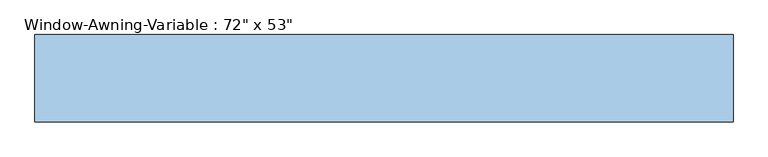
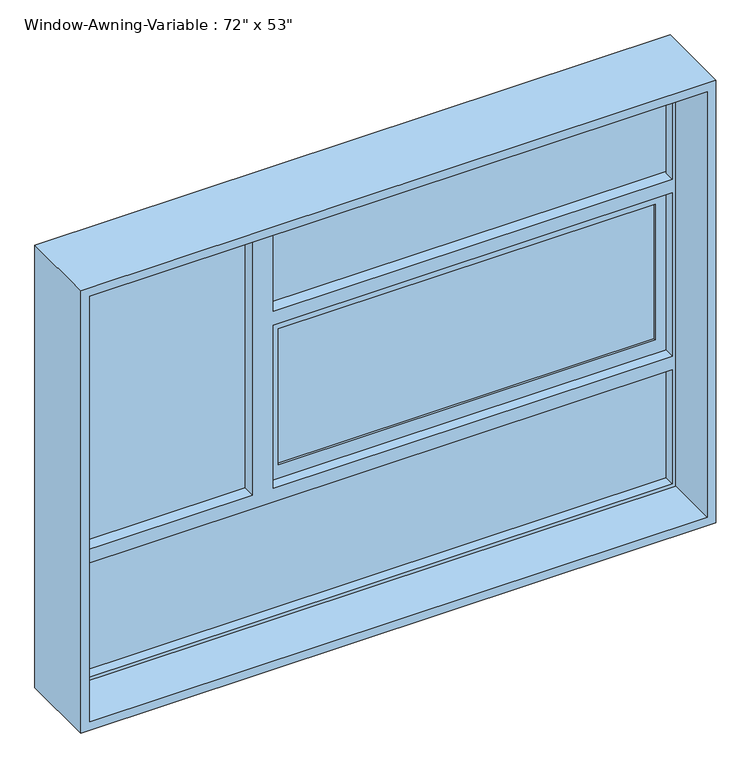
"""IFC4 building model written with IfcOpenShell, lengths in millimetres: window geometry."""

from ifc_helpers import new_model, si_unit, frame, origin, place, context, project, spatial, polyline, outline, extrude, faceted_brep, source, transform, mapped, element, save


def window_dd9b4f56(model_context):
    return source(origin(), model_context, "Body", "SolidModel", [
        extrude(outline(polyline([(847.1296875, 98.425), (847.1296875, 92.075), (-237.5296875, 92.075), (-237.5296875, 98.425), (847.1296875, 98.425)])), frame((0.0, 0.0, 1381.0654688), z_axis=(0.0, 0.0, 1.0), x_axis=(1.0, 0.0, 0.0)), (0.0, 0.0, 1.0), 412.8690625),
        extrude(outline(polyline([(847.1296875, 85.725), (847.1296875, 79.375), (-237.5296875, 79.375), (-237.5296875, 85.725), (847.1296875, 85.725)])), frame((0.0, 0.0, 1381.0654688), z_axis=(0.0, 0.0, 1.0), x_axis=(1.0, 0.0, 0.0)), (0.0, 0.0, 1.0), 412.8690625),
        extrude(outline(polyline([(-330.2, 98.425), (-330.2, 92.075), (-889.0, 92.075), (-889.0, 98.425), (-330.2, 98.425)])), frame((0.0, 0.0, 1339.1951563), z_axis=(0.0, 0.0, 1.0), x_axis=(1.0, 0.0, 0.0)), (0.0, 0.0, 1.0), 896.0048438),
        extrude(outline(polyline([(-330.2, 85.725), (-330.2, 79.375), (-889.0, 79.375), (-889.0, 85.725), (-330.2, 85.725)])), frame((0.0, 0.0, 1339.1951563), z_axis=(0.0, 0.0, 1.0), x_axis=(1.0, 0.0, 0.0)), (0.0, 0.0, 1.0), 896.0048438),
        extrude(outline(polyline([(889.0, 85.725), (889.0, 79.375), (-279.4, 79.375), (-279.4, 85.725), (889.0, 85.725)])), frame((0.0, 0.0, 1877.6751563), z_axis=(0.0, 0.0, 1.0), x_axis=(1.0, 0.0, 0.0)), (0.0, 0.0, 1.0), 357.5248438),
        extrude(outline(polyline([(889.0, 98.425), (889.0, 92.075), (-279.4, 92.075), (-279.4, 98.425), (889.0, 98.425)])), frame((0.0, 0.0, 1877.6751563), z_axis=(0.0, 0.0, 1.0), x_axis=(1.0, 0.0, 0.0)), (0.0, 0.0, 1.0), 357.5248438),
        extrude(outline(polyline([(889.0, 98.425), (889.0, 92.075), (-889.0, 92.075), (-889.0, 98.425), (889.0, 98.425)])), frame((0.0, 0.0, 939.8), z_axis=(0.0, 0.0, 1.0), x_axis=(1.0, 0.0, 0.0)), (0.0, 0.0, 1.0), 357.5248438),
        extrude(outline(polyline([(889.0, 85.725), (889.0, 79.375), (-889.0, 79.375), (-889.0, 85.725), (889.0, 85.725)])), frame((0.0, 0.0, 939.8), z_axis=(0.0, 0.0, 1.0), x_axis=(1.0, 0.0, 0.0)), (0.0, 0.0, 1.0), 357.5248438),
        faceted_brep([(-889.0, 73.025, 2235.2), (-889.0, 114.3, 2235.2), (889.0, 114.3, 2235.2), (889.0, 73.025, 2235.2), (-279.4, 73.025, 2235.2), (-279.4, 111.125, 2235.2), (-330.2, 111.125, 2235.2), (-330.2, 73.025, 2235.2), (-878.8796875, 42.06875, 2225.0796875), (-878.8796875, 73.025, 2225.0796875), (-330.2, 73.025, 2225.0796875), (-330.2, 42.06875, 2225.0796875), (878.8796875, 73.025, 2225.0796875), (878.8796875, 42.06875, 2225.0796875), (-269.2796875, 42.06875, 2225.0796875), (-269.2796875, 73.025, 2225.0796875), (-889.0, -114.3, 2235.2), (-889.0, 42.06875, 2235.2), (889.0, 42.06875, 2235.2), (889.0, -114.3, 2235.2), (-914.4, 114.3, 2260.6), (-914.4, -114.3, 2260.6), (914.4, -114.3, 2260.6), (914.4, 114.3, 2260.6), (889.0, 114.3, 939.8), (889.0, 73.025, 939.8), (889.0, 73.025, 1297.3248438), (889.0, 111.125, 1297.3248438), (889.0, 111.125, 1339.1951563), (889.0, 73.025, 1339.1951563), (889.0, 73.025, 1835.8048438), (889.0, 111.125, 1835.8048438), (889.0, 111.125, 1877.6751563), (889.0, 73.025, 1877.6751563), (878.8796875, 73.025, 1877.6751563), (878.8796875, 42.06875, 1877.6751563), (878.8796875, 73.025, 949.9203125), (878.8796875, 42.06875, 949.9203125), (878.8796875, 42.06875, 1297.3248438), (878.8796875, 73.025, 1297.3248438), (878.8796875, 73.025, 1339.1951563), (878.8796875, 42.06875, 1339.1951563), (878.8796875, 42.06875, 1835.8048438), (878.8796875, 73.025, 1835.8048438), (889.0, 42.06875, 939.8), (889.0, -114.3, 939.8), (914.4, -114.3, 914.4), (914.4, 114.3, 914.4), (-889.0, 114.3, 939.8), (-889.0, 73.025, 939.8), (-878.8796875, 73.025, 949.9203125), (-878.8796875, 42.06875, 949.9203125), (-889.0, 42.06875, 939.8), (-889.0, -114.3, 939.8), (-914.4, -114.3, 914.4), (-914.4, 114.3, 914.4), (-889.0, 73.025, 1339.1951563), (-889.0, 111.125, 1339.1951563), (-889.0, 111.125, 1297.3248438), (-889.0, 73.025, 1297.3248438), (-269.2796875, 73.025, 1877.6751563), (-279.4, 73.025, 1877.6751563), (-878.8796875, 73.025, 1297.3248438), (-878.8796875, 73.025, 1339.1951563), (-269.2796875, 73.025, 1339.1951563), (-279.4, 73.025, 1339.1951563), (-279.4, 73.025, 1835.8048438), (-269.2796875, 73.025, 1835.8048438), (-878.8796875, 42.06875, 1339.1951563), (-878.8796875, 42.06875, 1297.3248438), (-269.2796875, 42.06875, 1877.6751563), (-330.2, 42.06875, 1339.1951563), (-269.2796875, 42.06875, 1339.1951563), (-269.2796875, 42.06875, 1835.8048438), (-330.2, 111.125, 1339.1951563), (-279.4, 111.125, 1877.6751563), (-279.4, 111.125, 1835.8048438), (-279.4, 111.125, 1339.1951563)], [[[0, 1, 2, 3, 4, 5, 6, 7]], [[8, 9, 10, 11]], [[12, 13, 14, 15]], [[16, 17, 18, 19]], [[20, 21, 22, 23]], [[3, 2, 24, 25, 26, 27, 28, 29, 30, 31, 32, 33]], [[13, 12, 34, 35]], [[36, 37, 38, 39]], [[40, 41, 42, 43]], [[19, 18, 44, 45]], [[23, 22, 46, 47]], [[25, 24, 48, 49]], [[37, 36, 50, 51]], [[45, 44, 52, 53]], [[47, 46, 54, 55]], [[1, 0, 56, 57, 58, 59, 49, 48]], [[12, 15, 60, 61, 4, 3, 33, 34]], [[25, 49, 59, 62, 50, 36, 39, 26]], [[56, 0, 7, 10, 9, 63]], [[29, 40, 43, 30]], [[64, 65, 66, 67]], [[9, 8, 68, 63]], [[51, 50, 62, 69]], [[52, 44, 18, 17], [14, 13, 35, 70], [37, 51, 69, 38], [68, 8, 11, 71], [72, 73, 42, 41]], [[17, 16, 53, 52]], [[22, 21, 54, 46], [16, 19, 45, 53]], [[21, 20, 55, 54]], [[20, 23, 47, 55], [2, 1, 48, 24]], [[58, 27, 26, 39, 38, 69, 62, 59]], [[27, 58, 57, 74, 6, 5, 75, 32, 31, 76, 77, 28]], [[29, 28, 77, 65, 64, 72, 41, 40]], [[57, 56, 63, 68, 71, 74]], [[6, 74, 71, 11, 10, 7]], [[15, 14, 70, 60]], [[72, 64, 67, 73]], [[5, 4, 61, 75]], [[65, 77, 76, 66]], [[76, 31, 30, 43, 42, 73, 67, 66]], [[32, 75, 61, 60, 70, 35, 34, 33]]]),
        extrude(outline(polyline([(1339.1951563, -279.4), (1339.1951563, 889.0), (1835.8048438, 889.0), (1835.8048438, -279.4), (1339.1951563, -279.4)]), holes=[polyline([(1381.0654688, -237.5296875), (1793.9345313, -237.5296875), (1793.9345313, 847.1296875), (1381.0654688, 847.1296875), (1381.0654688, -237.5296875)])]), frame((0.0, 73.025, 0.0), z_axis=(0.0, 1.0, 0.0), x_axis=(0.0, 0.0, 1.0)), (0.0, 0.0, 1.0), 31.75),
    ])


if __name__ == "__main__":
    model = new_model("IFC4")
    model_context = context("Model", 3, world=origin())
    ifc_project = project(units=[si_unit("LENGTHUNIT", "METRE", prefix="MILLI")], contexts=[model_context])
    site = spatial("IfcSite", under=ifc_project)
    building = spatial("IfcBuilding", under=site)
    placement = place(None, origin())
    window_shape = window_dd9b4f56(model_context)
    element("IfcWindow", 1, ObjectType="Window-Awning-Variable : 72\" x 53\"", at=placement, inside=building, context=model_context, shape_type="MappedRepresentation", body=[
        mapped(window_shape, transform((0.0, 0.0, 0.0), x_axis=(1.0, 0.0, 0.0), y_axis=(0.0, 1.0, 0.0), z_axis=(0.0, 0.0, 1.0))),
    ])
    save(model, "model.ifc")

# Revit data of these elements
# Type "Window-Awning-Variable : 72\" x 53\""
#   Type Mark = "39"
#   Fire Rating = "0.5h"
#   Assembly Code = "B2020100"
#   Analytic Construction = "Double glazing - domestic"
#   Window Inset [instance default] = 0' - 0 5/8"
#   Wall Thickness [instance default] = 0' - 6"
#   Visual Light Transmittance = 0.81
#   Transom Height Ratio = 0.3
#   Transom Height = 1' - 3.9"
#   Thermal Resistance (R) = 1.8146 (h·ft²·°F)/BTU
#   Solar Heat Gain Coefficient = 0.76
#   Rough Width = 6' - 0 1/2"
#   Rough Height = 4' - 5 1/2"
#   Opening Window Width = 4' - 0"
#   Opening Window Height = 1' - 9.2"
#   Heat Transfer Coefficient (U) = 0.5511 BTU/(h·ft²·°F)
#   Height = 4' - 5"
#   Frame Gap 3 [instance default] = 0' - 1 83/128"
#   Frame Gap 2 [instance default] = 0' - 0 5/8"
#   Frame Gap 1 = 0' - 1 51/128"
#   Fixed Window Width = 2' - 0"
#   Default Sill Height = 3' - 0"
#   Width = 6' - 0"
#   Frame Material = Metal - Aluminum
#   Glass Panel Material = Glass
#   Wall Closure = (empty or 0)
# Element 1 (IfcWindow, "Window-Awning-Variable : 72\" x 53\"")
#   Wall Thickness = 0' - 9"
#   Materials on its faces: "Glass", "Metal - Aluminum"
# Materials
#   "Metal - Aluminum": class "Metal", colour RGB 247 247 247, transparency 0
#   "Glass": class "Glass", colour RGB 0 128 192, transparency 0.75, Description = "Soda Lime Glass", Cost = 0
